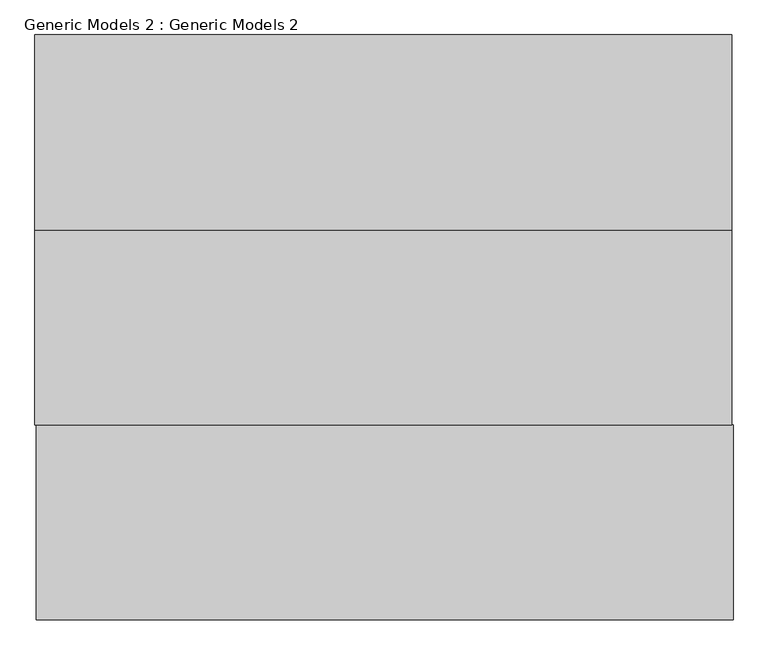
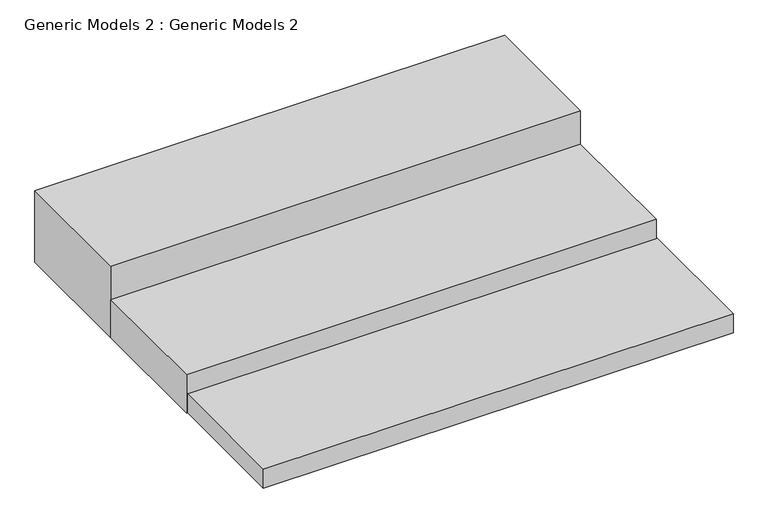
"""IFC4 building model written with IfcOpenShell, lengths in millimetres: proxy geometry, Generic Models 2 : Generic Models 2."""

from ifc_helpers import new_model, si_unit, origin, origin_with_axes, place, context, project, spatial, polyline, outline, extrude, source, transform, mapped, element, save


def generic_models_2_generic_models_2_51d3bdcd(model_context):
    return source(origin(), model_context, "Body", "SweptSolid", [
        extrude(outline(polyline([(3597.890657, 2398.4638821), (3597.890657, 2067.3458232), (2415.1418923, 2067.3458232), (2415.1418923, 2398.4638821), (3597.890657, 2398.4638821)])), origin_with_axes(), (0.0, 0.0, 1.0), 50.6317014),
        extrude(outline(polyline([(3595.7487647, 2729.5819411), (3595.7487647, 2398.4638821), (2413.0, 2398.4638821), (2413.0, 2729.5819411), (3595.7487647, 2729.5819411)])), origin_with_axes(), (0.0, 0.0, 1.0), 101.9801398),
        extrude(outline(polyline([(3595.7487647, 3060.7), (3595.7487647, 2729.5819411), (2413.0, 2729.5819411), (2413.0, 3060.7), (3595.7487647, 3060.7)])), origin_with_axes(), (0.0, 0.0, 1.0), 190.9934673),
    ])


if __name__ == "__main__":
    model = new_model("IFC4")
    model_context = context("Model", 3, world=origin())
    ifc_project = project(units=[si_unit("LENGTHUNIT", "METRE", prefix="MILLI")], contexts=[model_context])
    site = spatial("IfcSite", under=ifc_project)
    building = spatial("IfcBuilding", under=site)
    placement = place(None, origin())
    generic_models_2_generic_models_2_shape = generic_models_2_generic_models_2_51d3bdcd(model_context)
    element("IfcBuildingElementProxy", 1, Name="Generic Models 2 : Generic Models 2", ObjectType="Generic Models 2 : Generic Models 2", at=placement, inside=building, context=model_context, shape_type="MappedRepresentation", body=[
        mapped(generic_models_2_generic_models_2_shape, transform((0.0, 0.0, 0.0), x_axis=(1.0, 0.0, 0.0), y_axis=(0.0, 1.0, 0.0), z_axis=(0.0, 0.0, 1.0))),
    ])
    save(model, "model.ifc")

# Revit data of these elements
# Element 1 (IfcBuildingElementProxy, "Generic Models 2 : Generic Models 2")
#   Materials on its faces: "Cherry"
# Materials
#   "Cherry": class "Wood", colour RGB 226 177 128, transparency 0, Description = "Prunus Serotina", Cost = 0
